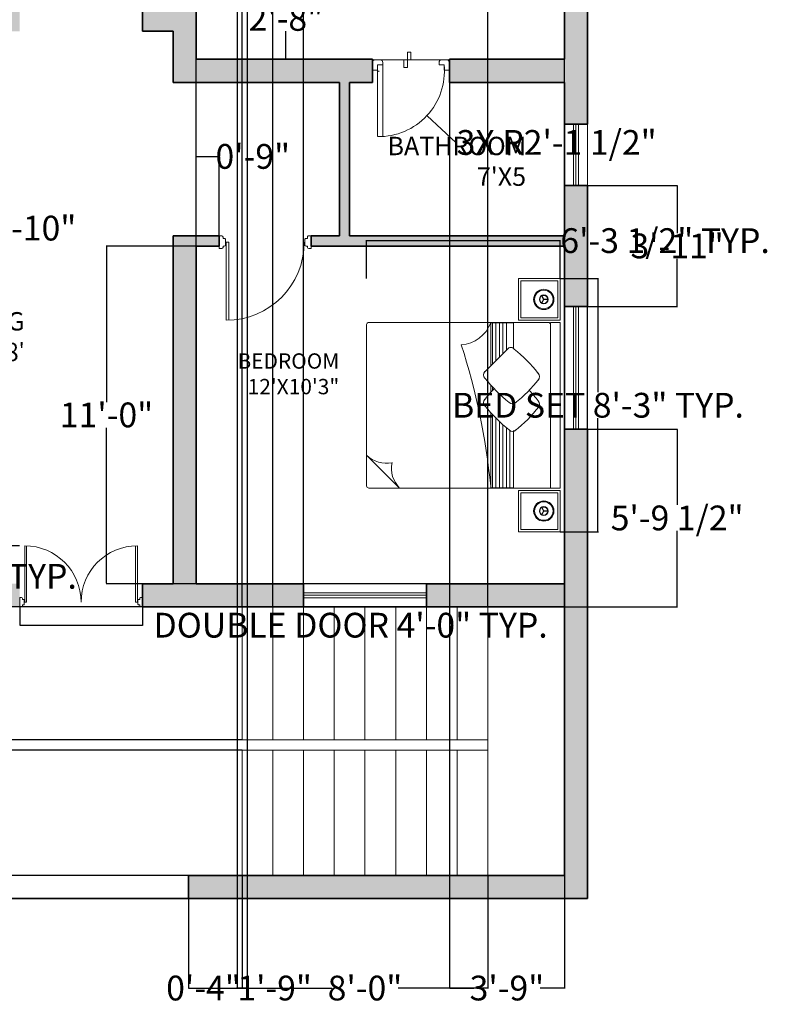
# Model space of a CAD drawing. Units: inches. Extents: x 2103 to 2702, y 2405 to 3142.
# Tile 2 of 7: x 2384 to 2677, y 2405 to 2790. Entities that reach past the tile are written whole.
import ezdxf

# ---------------------------------------------------------------- set-up
doc = ezdxf.new("R2010")
doc.units = ezdxf.units.IN
doc.linetypes.add('0', pattern=[0])
for name, color, linetype, lineweight in [('00 FURNITURE', 15, 'Continuous', 15), ('A-ANNO-DIMS', 2, 'Continuous', 18), ('A-AREA-IDEN', 7, 'Continuous', 18), ('A-FLOR-STRS', 7, 'Continuous', 18), ('A-WALL-PATT', 8, 'Continuous', 9), ('A_FUR 1', 5, 'Continuous', 5), ('doors', 4, 'Continuous', 18), ('WALL', 7, 'Continuous', 35), ('WINDOW', 160, '0', 5), ('windows', 4, 'Continuous', 18)]:
    doc.layers.add(name, color=color, linetype=linetype, lineweight=lineweight)
doc.layers.add('furniture', color=34, linetype='Continuous')
doc.styles.get("Standard").update_dxf_attribs({"font": 'arial.ttf'})
doc.dimstyles.get("Standard").update_dxf_attribs({"dimtxt": 9.68, "dimasz": 0.18, "dimexe": 0.18, "dimexo": 0.0625, "dimgap": 0.09, "dimtad": 0, "dimtih": 1, "dimtoh": 1, "dimdec": 1, "dimzin": 0, "dimdsep": 46, "dimlunit": 3, "dimtxsty": 'Standard', "dimcen": 0.09, "dimadec": 0, "dimazin": 0, "dimtfac": 1, "dimtdec": 1, "dimtofl": 0, "dimtmove": 0, "dimatfit": 3, "dimfxl": 1, "dimtolj": 1, "dimtzin": 0, "dimarcsym": 0})

# ---------------------------------------------------------------- blocks, each defined once
blk = doc.blocks.new('ESTSET')
at = {"layer": 'A_FUR 1'}
for p, q in [((-10.44, 4.1), (-10.44, 32.1)), ((-8.44, 4.1), (-8.44, 32.1)), ((-36.44, 6.1), (-36.44, 3.1)), ((-34.44, 6.1), (-36.44, 6.1)), ((-34.44, 4.1), (-34.44, 6.1)), ((-34.44, 4.1), (-34.44, 6.1)), ((-32.44, 4.1), (-34.44, 4.1)), ((-32.44, 4.1), (-34.44, 4.1)), ((-32.44, 3.1), (-32.44, 4.1)), ((-10.44, 3.1), (-10.44, 4.1)), ((-10.44, 4.1), (-8.44, 4.1)), ((-10.44, 4.1), (-8.44, 4.1)), ((-8.44, 4.1), (-8.44, 6.1)), ((-8.44, 6.1), (-6.44, 6.1)), ((-8.44, 4.1), (-8.44, 6.1)), ((-6.44, 6.1), (-6.44, 3.1)), ((-6.44, 2.1), (-36.44, 2.1)), ((-35.44, 2.1), (-33.44, 2.1)), ((-7.44, 2.1), (-9.44, 2.1))]:
    blk.add_line(p, q, dxfattribs=at)
for points in [[(-21.44, 2.1), (-18.67, 2.1), (-18.67, 5.1), (-20.06, 5.1)], [(-20.06, 5.1), (-20.06, -0.91)], [(-21.44, 2.1), (-21.44, -0.91), (-20.06, -0.91)]]:
    blk.add_lwpolyline(points, dxfattribs=at)
for centre, radius, start, end in [((-8.91, 6.46), 25.64, 88.9606, 185.2816), ((-35.44, 3.1), 1, 180, 270), ((-33.44, 3.1), 1, 270, 0), ((-9.44, 3.1), 1, 180, 270), ((-7.44, 3.1), 1, 270, 0)]:
    blk.add_arc(centre, radius, start, end, dxfattribs=at)
blk = doc.blocks.new('PUJA')
at = {"layer": '00 FURNITURE'}
for p, q in [((-1940.35, -16093.35), (-1958.14, -16093.35)), ((-1940.35, -16093.93), (-1958.13, -16093.93)), ((-1941.8, -16091.75), (-1938.89, -16091.75)), ((-1941.8, -16092.33), (-1941.8, -16091.75)), ((-1941.22, -16092.62), (-1941.51, -16092.62)), ((-1940.35, -16093.35), (-1940.35, -16093.93)), ((-1939.18, -16092.62), (-1939.47, -16092.62)), ((-1938.89, -16091.75), (-1938.89, -16092.33)), ((-1940.35, -16128.35), (-1958.13, -16128.35)), ((-1940.35, -16128.93), (-1940.35, -16128.35)), ((-1940.35, -16128.93), (-1958.14, -16128.93)), ((-1941.8, -16129.96), (-1941.8, -16130.54)), ((-1941.8, -16130.54), (-1938.89, -16130.54)), ((-1941.22, -16129.66), (-1941.51, -16129.66)), ((-1939.18, -16129.66), (-1939.47, -16129.66)), ((-1938.89, -16130.54), (-1938.89, -16129.96))]:
    blk.add_line(p, q, dxfattribs=at)
for points in [[(-1939.47, -16092.62), (-1939.47, -16092.91, -0.414214), (-1939.76, -16093.21), (-1940.93, -16093.21, -0.414214), (-1941.22, -16092.91), (-1941.22, -16092.62)], [(-1939.47, -16129.66), (-1939.47, -16129.37, 0.414214), (-1939.76, -16129.08), (-1940.93, -16129.08, 0.414214), (-1941.22, -16129.37), (-1941.22, -16129.66)]]:
    blk.add_lwpolyline(points, format="xyb", dxfattribs=at)
for centre, radius, start, end in [((-1940.35, -16093.35), 17.79, 180, 270), ((-1941.51, -16092.33), 0.292, 180, 270), ((-1939.18, -16092.33), 0.292, 270, 0), ((-1940.35, -16128.93), 17.79, 90, 180), ((-1941.51, -16129.96), 0.292, 90, 180), ((-1939.18, -16129.96), 0.292, 0, 90)]:
    blk.add_arc(centre, radius, start, end, dxfattribs=at)
blk = doc.blocks.new('DDD')
at = {"layer": '00 FURNITURE'}
for p, q in [((-12579.77, -15859.53), (-12579.77, -15829.05)), ((-12578.77, -15859.53), (-12578.77, -15829.03)), ((-12612.02, -15857.03), (-12612.02, -15862.03)), ((-12611.02, -15857.03), (-12612.02, -15857.03)), ((-12610.52, -15858.03), (-12610.52, -15857.53)), ((-12577.52, -15858.03), (-12577.52, -15857.53)), ((-12577.02, -15857.03), (-12576.02, -15857.03)), ((-12576.02, -15857.03), (-12576.02, -15862.03)), ((-12610.52, -15861.53), (-12610.52, -15861.03)), ((-12578.77, -15859.53), (-12579.77, -15859.53)), ((-12577.52, -15861.53), (-12577.52, -15861.03)), ((-12612.02, -15862.03), (-12611.02, -15862.03)), ((-12576.02, -15862.03), (-12577.02, -15862.03))]:
    blk.add_line(p, q, dxfattribs=at)
for points in [[(-12610.52, -15861.03), (-12610.02, -15861.03, 0.414214), (-12609.52, -15860.53), (-12609.52, -15858.53, 0.414214), (-12610.02, -15858.03), (-12610.52, -15858.03)], [(-12577.52, -15861.03), (-12578.02, -15861.03, -0.414214), (-12578.52, -15860.53), (-12578.52, -15858.53, -0.414214), (-12578.02, -15858.03), (-12577.52, -15858.03)]]:
    blk.add_lwpolyline(points, format="xyb", dxfattribs=at)
for centre, radius, start, end in [((-12578.77, -15859.53), 30.5, 90, 180), ((-12611.02, -15857.53), 0.5, 0, 90), ((-12577.02, -15857.53), 0.5, 90, 180), ((-12611.02, -15861.53), 0.5, 270, 0), ((-12577.02, -15861.53), 0.5, 180, 270)]:
    blk.add_arc(centre, radius, start, end, dxfattribs=at)
blk = doc.blocks.new('window')
at = {"layer": 'furniture'}
for p, q in [((1745.13, 2764.08), (1745.13, 2716.08)), ((1754.13, 2716.08), (1754.13, 2764.08))]:
    blk.add_line(p, q, dxfattribs=at)
at = {"layer": 'WINDOW'}
for p, q in [((1748.63, 2764.08), (1748.63, 2716.08)), ((1749.63, 2764.08), (1749.63, 2716.08)), ((1750.63, 2764.08), (1750.63, 2716.08))]:
    blk.add_line(p, q, dxfattribs=at)
blk = doc.blocks.new('ventilator')
at = {"layer": 'windows'}
for p, q in [((1922.12, 2523.05), (1898.12, 2523.05)), ((1922.12, 2522.05), (1898.12, 2522.05)), ((1922.12, 2521.05), (1898.12, 2521.05))]:
    blk.add_line(p, q, dxfattribs=at)
blk.add_lwpolyline([(1898.12, 2526.55), (1898.12, 2517.55), (1922.12, 2517.55), (1922.12, 2526.55)], close=True, dxfattribs=at)
blk = doc.blocks.new('RGWTG')
at = {"layer": '00 FURNITURE'}
for p, q in [((578.23, 3473.51), (577.36, 3475.01)), ((578.23, 3473.58), (577.36, 3472.08)), ((578.36, 3473.58), (577.49, 3475.09)), ((578.36, 3473.51), (577.49, 3472)), ((578.29, 3473.62), (580.03, 3473.62)), ((578.29, 3473.47), (580.03, 3473.47)), ((521.93, 3464.58), (509.03, 3451.68)), ((509.93, 3464.58), (566.4, 3464.58)), ((557.53, 3463.84), (557.53, 3464.49)), ((557.53, 3464.49), (566.4, 3464.49)), ((558.2, 3464.49), (558.2, 3435.82)), ((559.57, 3464.49), (559.57, 3437.25)), ((560.94, 3464.49), (560.94, 3438.58)), ((562.3, 3464.49), (562.3, 3439.83)), ((563.67, 3464.49), (563.67, 3440.99)), ((565.04, 3464.49), (565.04, 3442.08)), ((566.4, 3464.58), (580.98, 3464.58)), ((566.4, 3464.49), (566.4, 3442.08)), ((566.4, 3464.49), (566.4, 3463.84)), ((580.98, 3464.58), (580.98, 3416.72)), ((509.03, 3422.63), (509.03, 3463.68)), ((558.2, 3426.48), (558.2, 3425.04)), ((509.03, 3400.68), (509.03, 3422.63)), ((558.2, 3416.13), (558.2, 3399.95)), ((559.57, 3414.75), (559.57, 3399.95)), ((580.98, 3416.72), (580.98, 3400.68)), ((560.94, 3413.39), (560.94, 3399.95)), ((562.3, 3412.04), (562.3, 3399.95)), ((563.67, 3410.72), (563.67, 3399.95)), ((580.08, 3399.78), (509.93, 3399.78)), ((557.53, 3399.95), (557.53, 3400.6)), ((566.4, 3399.95), (557.53, 3399.95)), ((566.4, 3400.6), (566.4, 3399.95)), ((578.23, 3390.78), (577.36, 3392.29)), ((578.36, 3390.86), (577.49, 3392.36)), ((578.23, 3390.86), (577.36, 3389.36)), ((578.36, 3390.78), (577.49, 3389.28)), ((578.29, 3390.9), (580.03, 3390.9)), ((578.29, 3390.74), (580.03, 3390.74))]:
    blk.add_line(p, q, dxfattribs=at)
for points in [[(568.43, 3465.48), (584.63, 3465.48), (584.63, 3481.68), (568.43, 3481.68)], [(569.33, 3466.38), (583.73, 3466.38), (583.73, 3480.78), (569.33, 3480.78)], [(580.98, 3399.78), (584.63, 3399.78), (584.63, 3464.58), (580.98, 3464.58)], [(568.43, 3398.88), (584.63, 3398.88), (584.63, 3382.68), (568.43, 3382.68)], [(569.33, 3397.98), (583.73, 3397.98), (583.73, 3383.58), (569.33, 3383.58)]]:
    blk.add_lwpolyline(points, close=True, dxfattribs=at)
for points in [[(566.52, 3464.49), (557.53, 3464.49), (557.53, 3435.08)], [(557.53, 3427.21), (557.53, 3424.3)], [(557.53, 3416.82), (557.53, 3399.95), (566.4, 3399.95), (566.4, 3409.94)]]:
    blk.add_lwpolyline(points, dxfattribs=at)
for centre, radius in [((578.29, 3473.54), 3.97), ((578.29, 3473.54), 3.63), ((578.29, 3473.54), 1.74), ((578.29, 3473.54), 1.56), ((578.29, 3390.82), 3.97), ((578.29, 3390.82), 3.63), ((578.29, 3390.82), 1.74), ((578.29, 3390.82), 1.56)]:
    blk.add_circle(centre, radius, dxfattribs=at)
for centre, radius, start, end in [((509.93, 3463.68), 0.9, 90, 180), ((529.65, 3456.88), 10.9, 135.0361, 191.9278), ((290.56, 3490.52), 268.3, 342.2214, 354.2925), ((516.73, 3443.97), 10.9, 78.0722, 134.9639), ((598.15, 3399.01), 54.32, 127.931, 142.069), ((566.05, 3440.57), 1.82, 45, 135), ((533.58, 3399.31), 54.32, 37.931, 52.069), ((556.59, 3431.11), 1.82, 135, 225), ((597.87, 3463.6), 54.32, 217.931, 224.141), ((598.15, 3388.23), 54.32, 127.931, 142.069), ((566.05, 3429.78), 1.82, 45, 135), ((533.58, 3388.53), 54.32, 37.931, 52.069), ((533.28, 3463.88), 54.32, 316.32, 322.069), ((574.84, 3431.77), 1.82, 315, 45), ((574.84, 3420.99), 1.82, 315, 45), ((556.59, 3420.33), 1.82, 135, 225), ((765.33, 3619.75), 290.45, 223.6069, 226.2326), ((533.28, 3453.1), 54.32, 307.931, 322.069), ((565.44, 3411.05), 1.47, 225.9674, 326.8337), ((545.02, 3395.29), 13.35, 20.4224, 85.5825), ((509.93, 3400.68), 0.9, 180, 270), ((580.08, 3400.68), 0.9, 270, 0)]:
    blk.add_arc(centre, radius, start, end, dxfattribs=at)
blk = doc.blocks.new('*D26')
at = {"layer": 'A-ANNO-DIMS', "color": 0, "lineweight": -2, "transparency": 16777216}
for p, q in [((2384.43, 2560.78), (2384.43, 2553.47)), ((2432.43, 2560.78), (2432.43, 2553.47)), ((2384.61, 2553.65), (2432.25, 2553.65)), ((2432.43, 2553.65), (2432.61, 2553.65))]:
    blk.add_line(p, q, dxfattribs=at)
at = {"layer": 'A-ANNO-DIMS', "color": 0, "transparency": 16777216}
for points in [[(2384.61, 2553.68), (2384.61, 2553.62), (2384.43, 2553.65)], [(2432.25, 2553.68), (2432.25, 2553.62), (2432.43, 2553.65)]]:
    blk.add_solid(points, dxfattribs=at)
at = {"layer": 'Defpoints', "color": 0, "transparency": 16777216}
for p in [(2384.43, 2560.85), (2432.43, 2560.85), (2432.43, 2553.65)]:
    blk.add_point(p, dxfattribs=at)
at = {"layer": 'A-ANNO-DIMS', "color": 0, "transparency": 16777216, "insert": (2513.81, 2553.65), "char_height": 9.68, "attachment_point": 5}
blk.add_mtext('\\A1;DOUBLE DOOR 4\'-0" TYP.', dxfattribs=at)
blk = doc.blocks.new('*D27')
at = {"layer": 'A-ANNO-DIMS', "color": 0, "lineweight": -2, "transparency": 16777216}
for p, q in [((2384.37, 2584.67), (2377.05, 2584.67)), ((2377.23, 2584.49), (2377.23, 2577.79)), ((2377.23, 2561.03), (2377.23, 2567.72)), ((2384.37, 2560.85), (2377.05, 2560.85))]:
    blk.add_line(p, q, dxfattribs=at)
at = {"layer": 'A-ANNO-DIMS', "color": 0, "transparency": 16777216}
for points in [[(2377.2, 2584.49), (2377.26, 2584.49), (2377.23, 2584.67)], [(2377.2, 2561.03), (2377.26, 2561.03), (2377.23, 2560.85)]]:
    blk.add_solid(points, dxfattribs=at)
at = {"layer": 'Defpoints', "color": 0, "transparency": 16777216}
for p in [(2384.43, 2584.67), (2377.23, 2560.85), (2384.43, 2560.85)]:
    blk.add_point(p, dxfattribs=at)
at = {"layer": 'A-ANNO-DIMS', "color": 0, "transparency": 16777216, "insert": (2377.23, 2572.76), "char_height": 9.68, "attachment_point": 5}
blk.add_mtext('\\A1;2\'-0" TYP.', dxfattribs=at)
blk = doc.blocks.new('*D28')
at = {"layer": 'A-ANNO-DIMS', "color": 0, "lineweight": -2, "transparency": 16777216}
for p, q in [((2595.74, 2689.13), (2610.71, 2689.13)), ((2610.53, 2688.95), (2610.53, 2644.73)), ((2610.53, 2590.31), (2610.53, 2634.53)), ((2595.74, 2590.13), (2610.71, 2590.13))]:
    blk.add_line(p, q, dxfattribs=at)
at = {"layer": 'A-ANNO-DIMS', "color": 0, "transparency": 16777216}
for points in [[(2610.5, 2688.95), (2610.56, 2688.95), (2610.53, 2689.13)], [(2610.5, 2590.31), (2610.56, 2590.31), (2610.53, 2590.13)]]:
    blk.add_solid(points, dxfattribs=at)
at = {"layer": 'Defpoints', "color": 0, "transparency": 16777216}
for p in [(2595.68, 2689.13), (2595.68, 2590.13), (2610.53, 2590.13)]:
    blk.add_point(p, dxfattribs=at)
at = {"layer": 'A-ANNO-DIMS', "color": 0, "transparency": 16777216, "insert": (2610.53, 2639.63), "char_height": 9.68, "attachment_point": 5}
blk.add_mtext('\\A1;BED SET 8\'-3" TYP.', dxfattribs=at)
blk = doc.blocks.new('*D29')
at = {"layer": 'A-ANNO-DIMS', "color": 0, "lineweight": -2, "transparency": 16777216}
for p, q in [((2520.08, 2689.19), (2520.08, 2704.16)), ((2520.26, 2703.98), (2595.5, 2703.98)), ((2595.68, 2689.19), (2595.68, 2704.16)), ((2595.68, 2703.98), (2595.86, 2703.98))]:
    blk.add_line(p, q, dxfattribs=at)
at = {"layer": 'A-ANNO-DIMS', "color": 0, "transparency": 16777216}
for points in [[(2520.26, 2704.01), (2520.26, 2703.95), (2520.08, 2703.98)], [(2595.5, 2704.01), (2595.5, 2703.95), (2595.68, 2703.98)]]:
    blk.add_solid(points, dxfattribs=at)
at = {"layer": 'Defpoints', "color": 0, "transparency": 16777216}
for p in [(2595.68, 2703.98), (2520.08, 2689.13), (2595.68, 2689.13)]:
    blk.add_point(p, dxfattribs=at)
at = {"layer": 'A-ANNO-DIMS', "color": 0, "transparency": 16777216, "insert": (2636.76, 2703.98), "char_height": 9.68, "attachment_point": 5}
blk.add_mtext('\\A1;6\'-3 1/2" TYP.', dxfattribs=at)
blk = doc.blocks.new('*D41')
at = {"layer": 'A-ANNO-DIMS', "color": 0, "lineweight": -2, "transparency": 16777216}
for p, q in [((2471.43, 2455.78), (2471.43, 2411.62)), ((2567.43, 2455.78), (2567.43, 2411.62)), ((2471.61, 2411.8), (2506.47, 2411.8)), ((2567.25, 2411.8), (2532.39, 2411.8))]:
    blk.add_line(p, q, dxfattribs=at)
at = {"layer": 'A-ANNO-DIMS', "color": 0, "transparency": 16777216}
for points in [[(2471.61, 2411.83), (2471.61, 2411.77), (2471.43, 2411.8)], [(2567.25, 2411.83), (2567.25, 2411.77), (2567.43, 2411.8)]]:
    blk.add_solid(points, dxfattribs=at)
at = {"layer": 'Defpoints', "color": 0, "transparency": 16777216}
for p in [(2471.43, 2455.85), (2567.43, 2455.85), (2567.43, 2411.8)]:
    blk.add_point(p, dxfattribs=at)
at = {"layer": 'A-ANNO-DIMS', "color": 0, "transparency": 16777216, "insert": (2519.43, 2411.8), "char_height": 9.68, "attachment_point": 5}
blk.add_mtext('\\A1;8\'-0"', dxfattribs=at)
blk = doc.blocks.new('*D42')
at = {"layer": 'A-ANNO-DIMS', "color": 0, "lineweight": -2, "transparency": 16777216}
for p, q in [((2471.37, 2504.85), (2211.2, 2504.85)), ((2211.38, 2504.67), (2211.38, 2485.3)), ((2211.38, 2456.03), (2211.38, 2475.4)), ((2471.37, 2455.85), (2211.2, 2455.85))]:
    blk.add_line(p, q, dxfattribs=at)
at = {"layer": 'A-ANNO-DIMS', "color": 0, "transparency": 16777216}
for points in [[(2211.35, 2504.67), (2211.41, 2504.67), (2211.38, 2504.85)], [(2211.35, 2456.03), (2211.41, 2456.03), (2211.38, 2455.85)]]:
    blk.add_solid(points, dxfattribs=at)
at = {"layer": 'Defpoints', "color": 0, "transparency": 16777216}
for p in [(2211.38, 2504.85), (2471.43, 2504.85), (2471.43, 2455.85)]:
    blk.add_point(p, dxfattribs=at)
at = {"layer": 'A-ANNO-DIMS', "color": 0, "transparency": 16777216, "insert": (2211.38, 2480.35), "char_height": 9.68, "attachment_point": 5}
blk.add_mtext('\\A1;4\'-1"', dxfattribs=at)
blk = doc.blocks.new('*D43')
at = {"layer": 'A-ANNO-DIMS', "color": 0, "lineweight": -2, "transparency": 16777216}
for p, q in [((2471.367635, 2560.845674), (2211.200134, 2560.845674)), ((2211.380134, 2560.665674), (2211.380134, 2539.775674)), ((2211.380134, 2509.025674), (2211.380134, 2529.915674)), ((2471.367635, 2508.845674), (2211.200134, 2508.845674))]:
    blk.add_line(p, q, dxfattribs=at)
at = {"layer": 'A-ANNO-DIMS', "color": 0, "transparency": 16777216}
for points in [[(2211.350134, 2560.665674), (2211.410134, 2560.665674), (2211.380134, 2560.845674)], [(2211.350134, 2509.025674), (2211.410134, 2509.025674), (2211.380134, 2508.845674)]]:
    blk.add_solid(points, dxfattribs=at)
at = {"layer": 'Defpoints', "color": 0, "transparency": 16777216}
for p in [(2211.380134, 2560.845674), (2471.430135, 2560.845674), (2471.430135, 2508.845674)]:
    blk.add_point(p, dxfattribs=at)
at = {"layer": 'A-ANNO-DIMS', "color": 0, "transparency": 16777216, "insert": (2211.380134, 2534.845674), "char_height": 9.68, "attachment_point": 5}
blk.add_mtext('\\A1;4\'-4"', dxfattribs=at)
blk = doc.blocks.new('*D44')
at = {"layer": 'A-ANNO-DIMS', "color": 0, "lineweight": -2, "transparency": 16777216}
for p, q in [((2471.43, 2560.91), (2471.43, 3118.9)), ((2471.61, 3118.72), (2483.25, 3118.72)), ((2483.43, 2560.91), (2483.43, 3118.9)), ((2483.43, 3118.72), (2483.61, 3118.72))]:
    blk.add_line(p, q, dxfattribs=at)
at = {"layer": 'A-ANNO-DIMS', "color": 0, "transparency": 16777216}
for points in [[(2471.61, 3118.75), (2471.61, 3118.69), (2471.43, 3118.72)], [(2483.25, 3118.75), (2483.25, 3118.69), (2483.43, 3118.72)]]:
    blk.add_solid(points, dxfattribs=at)
at = {"layer": 'Defpoints', "color": 0, "transparency": 16777216}
for p in [(2483.43, 3118.72), (2471.43, 2560.85), (2483.43, 2560.85)]:
    blk.add_point(p, dxfattribs=at)
at = {"layer": 'A-ANNO-DIMS', "color": 0, "transparency": 16777216, "insert": (2496.11, 3118.72), "char_height": 9.68, "attachment_point": 5}
blk.add_mtext('\\A1;1\'-0"', dxfattribs=at)
blk = doc.blocks.new('*D45')
at = {"layer": 'A-ANNO-DIMS', "color": 0, "lineweight": -2, "transparency": 16777216}
for p, q in [((2567.43, 2560.91), (2567.43, 3118.9)), ((2567.61, 3118.72), (2569.39, 3118.72)), ((2597.25, 3118.72), (2595.47, 3118.72)), ((2597.43, 2560.91), (2597.43, 3118.9))]:
    blk.add_line(p, q, dxfattribs=at)
at = {"layer": 'A-ANNO-DIMS', "color": 0, "transparency": 16777216}
for points in [[(2567.61, 3118.75), (2567.61, 3118.69), (2567.43, 3118.72)], [(2597.25, 3118.75), (2597.25, 3118.69), (2597.43, 3118.72)]]:
    blk.add_solid(points, dxfattribs=at)
at = {"layer": 'Defpoints', "color": 0, "transparency": 16777216}
for p in [(2597.43, 3118.72), (2567.43, 2560.85), (2597.43, 2560.85)]:
    blk.add_point(p, dxfattribs=at)
at = {"layer": 'A-ANNO-DIMS', "color": 0, "transparency": 16777216, "insert": (2582.43, 3118.72), "char_height": 9.68, "attachment_point": 5}
blk.add_mtext('\\A1;2\'-6"', dxfattribs=at)
blk = doc.blocks.new('*D46')
at = {"layer": 'A-ANNO-DIMS', "color": 0, "lineweight": -2, "transparency": 16777216}
for p, q in [((2450.43, 2455.78), (2450.43, 2411.62)), ((2471.43, 2455.78), (2471.43, 2411.62)), ((2450.61, 2411.8), (2471.25, 2411.8)), ((2471.43, 2411.8), (2471.61, 2411.8))]:
    blk.add_line(p, q, dxfattribs=at)
at = {"layer": 'A-ANNO-DIMS', "color": 0, "transparency": 16777216}
for points in [[(2450.61, 2411.83), (2450.61, 2411.77), (2450.43, 2411.8)], [(2471.25, 2411.83), (2471.25, 2411.77), (2471.43, 2411.8)]]:
    blk.add_solid(points, dxfattribs=at)
at = {"layer": 'Defpoints', "color": 0, "transparency": 16777216}
for p in [(2450.43, 2455.85), (2471.43, 2455.85), (2471.43, 2411.8)]:
    blk.add_point(p, dxfattribs=at)
at = {"layer": 'A-ANNO-DIMS', "color": 0, "transparency": 16777216, "insert": (2484.11, 2411.8), "char_height": 9.68, "attachment_point": 5}
blk.add_mtext('\\A1;1\'-9"', dxfattribs=at)
blk = doc.blocks.new('*D47')
at = {"layer": 'A-ANNO-DIMS', "color": 0, "lineweight": -2, "transparency": 16777216}
for p, q in [((2471.37, 2508.85), (2211.2, 2508.85)), ((2211.38, 2508.85), (2211.38, 2509.03)), ((2211.38, 2509.03), (2211.56, 2509.03)), ((2211.38, 2505.03), (2211.38, 2508.67)), ((2471.37, 2504.85), (2211.2, 2504.85))]:
    blk.add_line(p, q, dxfattribs=at)
at = {"layer": 'A-ANNO-DIMS', "color": 0, "transparency": 16777216}
for points in [[(2211.35, 2508.67), (2211.41, 2508.67), (2211.38, 2508.85)], [(2211.35, 2505.03), (2211.41, 2505.03), (2211.38, 2504.85)]]:
    blk.add_solid(points, dxfattribs=at)
at = {"layer": 'Defpoints', "color": 0, "transparency": 16777216}
for p in [(2211.38, 2508.85), (2471.43, 2508.85), (2471.43, 2504.85)]:
    blk.add_point(p, dxfattribs=at)
at = {"layer": 'A-ANNO-DIMS', "color": 0, "transparency": 16777216, "insert": (2224.52, 2509.03), "char_height": 9.68, "attachment_point": 5}
blk.add_mtext('\\A1;0\'-4"', dxfattribs=at)
blk = doc.blocks.new('*D50')
at = {"layer": 'A-ANNO-DIMS', "color": 0, "lineweight": -2, "transparency": 16777216}
for p, q in [((2453.43, 2569.91), (2453.43, 3118.9)), ((2453.61, 3118.72), (2461.48, 3118.72)), ((2495.25, 3118.72), (2487.38, 3118.72)), ((2495.43, 2569.91), (2495.43, 3118.9))]:
    blk.add_line(p, q, dxfattribs=at)
at = {"layer": 'A-ANNO-DIMS', "color": 0, "transparency": 16777216}
for points in [[(2453.61, 3118.75), (2453.61, 3118.69), (2453.43, 3118.72)], [(2495.25, 3118.75), (2495.25, 3118.69), (2495.43, 3118.72)]]:
    blk.add_solid(points, dxfattribs=at)
at = {"layer": 'Defpoints', "color": 0, "transparency": 16777216}
for p in [(2495.43, 3118.72), (2453.43, 2569.85), (2495.43, 2569.85)]:
    blk.add_point(p, dxfattribs=at)
at = {"layer": 'A-ANNO-DIMS', "color": 0, "transparency": 16777216, "insert": (2474.43, 3118.72), "char_height": 9.68, "attachment_point": 5}
blk.add_mtext('\\A1;3\'-6"', dxfattribs=at)
blk = doc.blocks.new('*D61')
at = {"layer": 'A-ANNO-DIMS', "color": 0, "lineweight": -2, "transparency": 16777216}
for p, q in [((2606.49, 2630.29), (2641.66, 2630.29)), ((2641.48, 2630.11), (2641.48, 2600.66)), ((2641.48, 2561.03), (2641.48, 2590.47)), ((2597.49, 2560.85), (2641.66, 2560.85))]:
    blk.add_line(p, q, dxfattribs=at)
at = {"layer": 'A-ANNO-DIMS', "color": 0, "transparency": 16777216}
for points in [[(2641.45, 2630.11), (2641.51, 2630.11), (2641.48, 2630.29)], [(2641.45, 2561.03), (2641.51, 2561.03), (2641.48, 2560.85)]]:
    blk.add_solid(points, dxfattribs=at)
at = {"layer": 'Defpoints', "color": 0, "transparency": 16777216}
for p in [(2606.43, 2630.29), (2641.48, 2630.29), (2597.43, 2560.85)]:
    blk.add_point(p, dxfattribs=at)
at = {"layer": 'A-ANNO-DIMS', "color": 0, "transparency": 16777216, "insert": (2641.48, 2595.57), "char_height": 9.68, "attachment_point": 5}
blk.add_mtext('\\A1;5\'-9 1/2"', dxfattribs=at)
blk = doc.blocks.new('*D62')
at = {"layer": 'A-ANNO-DIMS', "color": 0, "lineweight": -2, "transparency": 16777216}
for p, q in [((2606.49, 2725.52), (2641.66, 2725.52)), ((2641.48, 2725.34), (2641.48, 2706.94)), ((2641.48, 2678.47), (2641.48, 2696.87)), ((2606.49, 2678.29), (2641.66, 2678.29))]:
    blk.add_line(p, q, dxfattribs=at)
at = {"layer": 'A-ANNO-DIMS', "color": 0, "transparency": 16777216}
for points in [[(2641.45, 2725.34), (2641.51, 2725.34), (2641.48, 2725.52)], [(2641.45, 2678.47), (2641.51, 2678.47), (2641.48, 2678.29)]]:
    blk.add_solid(points, dxfattribs=at)
at = {"layer": 'Defpoints', "color": 0, "transparency": 16777216}
for p in [(2606.43, 2725.52), (2641.48, 2725.52), (2606.43, 2678.29)]:
    blk.add_point(p, dxfattribs=at)
at = {"layer": 'A-ANNO-DIMS', "color": 0, "transparency": 16777216, "insert": (2641.48, 2701.91), "char_height": 9.68, "attachment_point": 5}
blk.add_mtext('\\A1;3\'-11"', dxfattribs=at)
blk = doc.blocks.new('*D67')
at = {"layer": 'A-ANNO-DIMS', "color": 0, "lineweight": -2, "transparency": 16777216}
for p, q in [((2469.43, 2999.78), (2469.43, 2411.62)), ((2473.43, 2999.78), (2473.43, 2411.62)), ((2469.43, 2411.8), (2469.25, 2411.8)), ((2473.25, 2411.8), (2469.61, 2411.8))]:
    blk.add_line(p, q, dxfattribs=at)
at = {"layer": 'A-ANNO-DIMS', "color": 0, "transparency": 16777216}
for points in [[(2469.61, 2411.83), (2469.61, 2411.77), (2469.43, 2411.8)], [(2473.25, 2411.83), (2473.25, 2411.77), (2473.43, 2411.8)]]:
    blk.add_solid(points, dxfattribs=at)
at = {"layer": 'Defpoints', "color": 0, "transparency": 16777216}
for p in [(2469.43, 2999.85), (2473.43, 2999.85), (2469.43, 2411.8)]:
    blk.add_point(p, dxfattribs=at)
at = {"layer": 'A-ANNO-DIMS', "color": 0, "transparency": 16777216, "insert": (2456.29, 2411.8), "char_height": 9.68, "attachment_point": 5}
blk.add_mtext('\\A1;0\'-4"', dxfattribs=at)
blk = doc.blocks.new('*D71')
at = {"layer": 'A-ANNO-DIMS', "color": 0, "lineweight": -2, "transparency": 16777216}
for p, q in [((2453.49, 2806.85), (2488.66, 2806.85)), ((2488.48, 2806.67), (2488.48, 2795.88)), ((2488.48, 2775.03), (2488.48, 2785.81)), ((2453.49, 2774.85), (2488.66, 2774.85))]:
    blk.add_line(p, q, dxfattribs=at)
at = {"layer": 'A-ANNO-DIMS', "color": 0, "transparency": 16777216}
for points in [[(2488.45, 2806.67), (2488.51, 2806.67), (2488.48, 2806.85)], [(2488.45, 2775.03), (2488.51, 2775.03), (2488.48, 2774.85)]]:
    blk.add_solid(points, dxfattribs=at)
at = {"layer": 'Defpoints', "color": 0, "transparency": 16777216}
for p in [(2453.43, 2806.85), (2453.43, 2774.85), (2488.48, 2774.85)]:
    blk.add_point(p, dxfattribs=at)
at = {"layer": 'A-ANNO-DIMS', "color": 0, "transparency": 16777216, "insert": (2488.48, 2790.85), "char_height": 9.68, "attachment_point": 5}
blk.add_mtext('\\A1;2\'-8"', dxfattribs=at)
blk = doc.blocks.new('*D72')
at = {"layer": 'A-ANNO-DIMS', "color": 0, "lineweight": -2, "transparency": 16777216}
for p, q in [((2453.43, 2701.91), (2453.43, 2737.08)), ((2453.61, 2736.9), (2462.25, 2736.9)), ((2462.43, 2701.91), (2462.43, 2737.08)), ((2462.43, 2736.9), (2462.61, 2736.9))]:
    blk.add_line(p, q, dxfattribs=at)
at = {"layer": 'A-ANNO-DIMS', "color": 0, "transparency": 16777216}
for points in [[(2453.61, 2736.93), (2453.61, 2736.87), (2453.43, 2736.9)], [(2462.25, 2736.93), (2462.25, 2736.87), (2462.43, 2736.9)]]:
    blk.add_solid(points, dxfattribs=at)
at = {"layer": 'Defpoints', "color": 0, "transparency": 16777216}
for p in [(2462.43, 2736.9), (2453.43, 2701.85), (2462.43, 2701.85)]:
    blk.add_point(p, dxfattribs=at)
at = {"layer": 'A-ANNO-DIMS', "color": 0, "transparency": 16777216, "insert": (2475.57, 2736.9), "char_height": 9.68, "attachment_point": 5}
blk.add_mtext('\\A1;0\'-9"', dxfattribs=at)
blk = doc.blocks.new('*D73')
at = {"layer": 'A-ANNO-DIMS', "color": 0, "lineweight": -2, "transparency": 16777216}
for p, q in [((2552.43, 2765.78), (2552.43, 2411.62)), ((2597.43, 2765.78), (2597.43, 2411.62)), ((2552.61, 2411.8), (2561.98, 2411.8)), ((2597.25, 2411.8), (2587.88, 2411.8))]:
    blk.add_line(p, q, dxfattribs=at)
at = {"layer": 'A-ANNO-DIMS', "color": 0, "transparency": 16777216}
for points in [[(2552.61, 2411.83), (2552.61, 2411.77), (2552.43, 2411.8)], [(2597.25, 2411.83), (2597.25, 2411.77), (2597.43, 2411.8)]]:
    blk.add_solid(points, dxfattribs=at)
at = {"layer": 'Defpoints', "color": 0, "transparency": 16777216}
for p in [(2552.43, 2765.85), (2597.43, 2765.85), (2597.43, 2411.8)]:
    blk.add_point(p, dxfattribs=at)
at = {"layer": 'A-ANNO-DIMS', "color": 0, "transparency": 16777216, "insert": (2574.93, 2411.8), "char_height": 9.68, "attachment_point": 5}
blk.add_mtext('\\A1;3\'-9"', dxfattribs=at)
blk = doc.blocks.new('*D75')
at = {"layer": 'A-ANNO-DIMS', "color": 0, "lineweight": -2, "transparency": 16777216}
for p, q in [((2453.37, 2701.85), (2418.2, 2701.85)), ((2418.38, 2701.67), (2418.38, 2640.88)), ((2418.38, 2570.03), (2418.38, 2630.81)), ((2453.37, 2569.85), (2418.2, 2569.85))]:
    blk.add_line(p, q, dxfattribs=at)
at = {"layer": 'A-ANNO-DIMS', "color": 0, "transparency": 16777216}
for points in [[(2418.35, 2701.67), (2418.41, 2701.67), (2418.38, 2701.85)], [(2418.35, 2570.03), (2418.41, 2570.03), (2418.38, 2569.85)]]:
    blk.add_solid(points, dxfattribs=at)
at = {"layer": 'Defpoints', "color": 0, "transparency": 16777216}
for p in [(2418.38, 2701.85), (2453.43, 2701.85), (2453.43, 2569.85)]:
    blk.add_point(p, dxfattribs=at)
at = {"layer": 'A-ANNO-DIMS', "color": 0, "transparency": 16777216, "insert": (2418.38, 2635.85), "char_height": 9.68, "attachment_point": 5}
blk.add_mtext('\\A1;11\'-0"', dxfattribs=at)
blk = doc.blocks.new('*D78')
at = {"layer": 'A-ANNO-DIMS', "color": 0, "lineweight": -2, "transparency": 16777216}
for p, q in [((2342.12, 2708.86), (2342.3, 2708.86)), ((2342.21, 2708.77), (2342.21, 2708.95)), ((2359.73, 2708.87), (2353.34, 2708.86))]:
    blk.add_line(p, q, dxfattribs=at)
at = {"layer": 'A-ANNO-DIMS', "color": 0, "transparency": 16777216}
blk.add_solid([(2353.34, 2708.9), (2353.34, 2708.84), (2353.16, 2708.86)], dxfattribs=at)
at = {"layer": 'Defpoints', "color": 0, "transparency": 16777216}
for p in [(2331.26, 2708.86), (2353.16, 2708.86)]:
    blk.add_point(p, dxfattribs=at)
at = {"layer": 'A-ANNO-DIMS', "color": 0, "transparency": 16777216, "insert": (2381.71, 2708.87), "char_height": 9.68, "attachment_point": 5}
blk.add_mtext('\\A1;∅1\'-10"', dxfattribs=at)
blk = doc.blocks.new('*D80')
at = {"layer": 'A-ANNO-DIMS', "color": 0, "lineweight": -2, "transparency": 16777216}
for p, q in [((2524.77, 2770.28), (2524.95, 2770.28)), ((2524.86, 2770.19), (2524.86, 2770.37)), ((2554.93, 2742.36), (2543.79, 2752.71)), ((2555.11, 2742.36), (2554.93, 2742.36))]:
    blk.add_line(p, q, dxfattribs=at)
at = {"layer": 'A-ANNO-DIMS', "color": 0, "transparency": 16777216}
blk.add_solid([(2543.81, 2752.73), (2543.77, 2752.68), (2543.65, 2752.83)], dxfattribs=at)
at = {"layer": 'Defpoints', "color": 0, "transparency": 16777216}
for p in [(2524.86, 2770.28), (2543.65, 2752.83)]:
    blk.add_point(p, dxfattribs=at)
at = {"layer": 'A-ANNO-DIMS', "color": 0, "transparency": 16777216, "insert": (2594.37, 2742.36), "char_height": 9.68, "attachment_point": 5}
blk.add_mtext('\\A1;3X R2\'-1 1/2"', dxfattribs=at)

msp = doc.modelspace()

# ---------------------------------------------------------------- hatches: boundary and pattern name
at = {"layer": 'A-WALL-PATT'}
h = msp.add_hatch(color=256, dxfattribs=at)
h.dxf.hatch_style = 1
h.paths.add_polyline_path([(2342.43, 2911.85), (2342.43, 2915.85), (2255.43, 2915.85), (2255.43, 2976.23), (2246.43, 2976.23), (2246.43, 2840.19), (2255.43, 2840.19), (2255.43, 2854.85), (2315.43, 2854.85), (2315.43, 2845.85), (2319.43, 2845.85), (2319.43, 2858.85), (2255.43, 2858.85), (2255.43, 2906.85), (2342.43, 2906.85)])
h.paths.add_polyline_path([(2384.43, 2794.85), (2319.43, 2794.85), (2319.43, 2815.85), (2315.43, 2815.85), (2315.43, 2794.85), (2255.43, 2794.85), (2255.43, 2816.19), (2246.43, 2816.19), (2246.43, 2753.7), (2255.43, 2753.7), (2255.43, 2785.85), (2384.43, 2785.85)])
h.paths.add_polyline_path([(2606.43, 2963.85), (2597.43, 2963.85), (2597.43, 2951.85), (2537.43, 2951.85), (2537.43, 2957.85), (2533.43, 2957.85), (2533.43, 2951.85), (2469.43, 2951.85), (2444.43, 2951.85), (2444.43, 2842.85), (2449.43, 2842.85), (2453.43, 2842.85), (2453.43, 2942.85), (2597.43, 2942.85), (2597.43, 2904.89), (2606.43, 2904.89)])
h.paths.add_polyline_path([(2606.43, 3019.85), (2597.43, 3019.85), (2597.43, 3003.85), (2537.43, 3003.85), (2537.43, 3015.85), (2533.43, 3015.85), (2533.43, 2987.85), (2537.43, 2987.85), (2537.43, 2999.85), (2597.43, 2999.85), (2597.43, 2987.85), (2606.43, 2987.85)])
h.paths.add_polyline_path([(2606.43, 2856.89), (2597.43, 2856.89), (2597.43, 2774.85), (2552.43, 2774.85), (2552.43, 2765.85), (2597.43, 2765.85), (2597.43, 2749.52), (2606.43, 2749.52)])
h.paths.add_polyline_path([(2522.43, 2774.85), (2453.43, 2774.85), (2453.43, 2806.85), (2444.43, 2806.85), (2444.43, 2794.85), (2432.43, 2794.85), (2432.43, 2785.85), (2444.43, 2785.85), (2444.43, 2765.85), (2453.43, 2765.85), (2509.43, 2765.85), (2509.43, 2705.85), (2498.43, 2705.85), (2498.43, 2701.85), (2597.43, 2701.85), (2597.43, 2678.29), (2606.43, 2678.29), (2606.43, 2725.52), (2597.43, 2725.52), (2597.43, 2705.85), (2513.43, 2705.85), (2513.43, 2765.85), (2522.43, 2765.85)])
h.paths.add_polyline_path([(2255.43, 2705.7), (2246.43, 2705.7), (2246.43, 2646.55), (2255.43, 2646.55)])
h.paths.add_polyline_path([(2255.43, 2598.55), (2246.43, 2598.55), (2246.43, 2560.85), (2309.13, 2560.85), (2309.13, 2569.85), (2309.13, 2569.85), (2255.43, 2569.85)])
h.paths.add_polyline_path([(2495.43, 2569.85), (2495.43, 2569.85), (2453.43, 2569.85), (2453.43, 2701.85), (2462.43, 2701.85), (2462.43, 2705.85), (2444.43, 2705.85), (2444.43, 2569.85), (2432.43, 2569.85), (2432.43, 2564.45), (2432.43, 2564.45), (2432.43, 2560.85), (2495.43, 2560.85)])
h.paths.add_polyline_path([(2384.43, 2569.85), (2357.13, 2569.85), (2357.13, 2560.85), (2384.43, 2560.85)])
h.paths.add_polyline_path([(2606.43, 2630.29), (2597.43, 2630.29), (2597.43, 2569.85), (2543.43, 2569.85), (2543.43, 2560.85), (2597.43, 2560.85), (2597.43, 2455.85), (2450.43, 2455.85), (2450.43, 2446.85), (2606.43, 2446.85)])

# ---------------------------------------------------------------- linework, layer by layer
at = {"layer": 'A-FLOR-STRS'}
for p, q in [((2471.43, 2560.85), (2471.43, 2508.85)), ((2483.43, 2560.85), (2483.43, 2508.85)), ((2495.43, 2560.85), (2495.43, 2508.85)), ((2507.43, 2560.85), (2507.43, 2508.85)), ((2519.43, 2560.85), (2519.43, 2508.85)), ((2531.43, 2560.85), (2531.43, 2508.85)), ((2543.43, 2560.85), (2543.43, 2508.85)), ((2555.43, 2560.85), (2555.43, 2508.85)), ((2567.43, 2560.85), (2567.43, 2455.85)), ((2471.43, 2508.85), (2567.43, 2508.85)), ((2471.43, 2504.85), (2567.43, 2504.85)), ((2471.43, 2504.85), (2471.43, 2455.85)), ((2483.43, 2504.85), (2483.43, 2455.85)), ((2495.43, 2504.85), (2495.43, 2455.85)), ((2507.43, 2504.85), (2507.43, 2455.85)), ((2519.43, 2504.85), (2519.43, 2455.85)), ((2531.43, 2504.85), (2531.43, 2455.85)), ((2543.43, 2504.85), (2543.43, 2455.85)), ((2555.43, 2504.85), (2555.43, 2455.85))]:
    msp.add_line(p, q, dxfattribs=at)
at = {"layer": 'WALL'}
for p, q in [((2597.43, 2856.89), (2597.43, 2774.85)), ((2606.43, 2856.89), (2606.43, 2749.52)), ((2453.43, 2806.85), (2453.43, 2774.85)), ((2432.43, 2794.85), (2432.43, 2785.85)), ((2432.43, 2785.85), (2444.43, 2785.85)), ((2444.43, 2785.85), (2444.43, 2765.85)), ((2444.43, 2785.85), (2444.43, 2765.85)), ((2453.43, 2774.85), (2522.43, 2774.85)), ((2522.43, 2774.85), (2522.43, 2765.85)), ((2552.43, 2774.85), (2552.43, 2765.85)), ((2552.43, 2774.85), (2597.43, 2774.85)), ((2444.43, 2765.85), (2509.43, 2765.85)), ((2453.43, 2765.85), (2444.43, 2765.85)), ((2509.43, 2765.85), (2509.43, 2705.85)), ((2513.43, 2765.85), (2513.43, 2705.85)), ((2513.43, 2765.85), (2522.43, 2765.85)), ((2552.43, 2765.85), (2597.43, 2765.85)), ((2597.43, 2765.85), (2597.43, 2749.52)), ((2597.43, 2749.52), (2606.43, 2749.52)), ((2597.43, 2725.52), (2606.43, 2725.52)), ((2597.43, 2725.52), (2597.43, 2705.85)), ((2606.43, 2725.52), (2606.43, 2678.29)), ((2444.43, 2705.85), (2462.43, 2705.85)), ((2453.43, 2705.85), (2444.43, 2705.85)), ((2444.43, 2705.85), (2444.43, 2569.85)), ((2444.43, 2705.85), (2444.43, 2569.85)), ((2462.43, 2705.85), (2462.43, 2701.85)), ((2498.43, 2705.85), (2498.43, 2701.85)), ((2498.43, 2705.85), (2509.43, 2705.85)), ((2513.43, 2705.85), (2597.43, 2705.85)), ((2453.43, 2701.85), (2462.43, 2701.85)), ((2453.43, 2701.85), (2453.43, 2569.85)), ((2498.43, 2701.85), (2597.43, 2701.85)), ((2597.43, 2701.85), (2597.43, 2678.29)), ((2597.43, 2678.29), (2606.43, 2678.29)), ((2597.43, 2630.29), (2606.43, 2630.29)), ((2597.43, 2630.29), (2597.43, 2569.85)), ((2606.43, 2630.29), (2606.43, 2446.85)), ((2432.43, 2569.85), (2432.43, 2560.85)), ((2432.43, 2569.85), (2444.43, 2569.85)), ((2453.43, 2569.85), (2495.43, 2569.85)), ((2495.43, 2560.85), (2495.43, 2569.85)), ((2543.43, 2560.85), (2543.43, 2569.85)), ((2543.43, 2569.85), (2597.43, 2569.85)), ((2432.43, 2560.85), (2597.43, 2560.85)), ((2597.43, 2560.85), (2597.43, 2455.85)), ((2450.43, 2455.85), (2450.43, 2446.85)), ((2597.43, 2455.85), (2450.43, 2455.85)), ((2606.43, 2446.85), (2246.43, 2446.85))]:
    msp.add_line(p, q, dxfattribs=at)

# ---------------------------------------------------------------- block references
at = {"layer": '00 FURNITURE', "xscale": -1, "rotation": 180}
msp.add_blockref('RGWTG', (2011.05, 6071.81), dxfattribs=at)
at = {"layer": 'doors'}
for name, p, rotation in [('ESTSET', (2515.95, 2776.74), 180), ('DDD', (-10113.59, -13156.18), 179.9999999934867)]:
    msp.add_blockref(name, p, dxfattribs=dict(at, rotation=rotation))
at = {"layer": 'doors', "xscale": 1.237379162154587, "yscale": 1.237379162154587, "zscale": 1.237379162154587, "rotation": 270.0000000034012}
msp.add_blockref('PUJA', (22344.02, 161.71), dxfattribs=at)
at = {"layer": 'windows'}
for name, p, rotation in [('ventilator', (79.88, 4647.64), 270), ('window', (4351.56, 5394.37), 180), ('window', (-220.65, 4314.97), 270)]:
    msp.add_blockref(name, p, dxfattribs=dict(at, rotation=rotation))

# ---------------------------------------------------------------- texts
at = {"layer": 'A-AREA-IDEN', "attachment_point": 3}
for s, insert, char_height in [("BATHROOM\\P7'X5", (2582.41, 2744.57), 7.188), ('LIVING \\P15\'9"X18{\\H0.83478x;\'}', (2386.33, 2676.03), 7.1875), (' {\\H0.83478x;BEDROOM  12\'X10\'3"}', (2509.39, 2659.92), 7.1875)]:
    msp.add_mtext_dynamic_manual_height_columns(s, width=41.3807, gutter_width=12.5, heights=[0], dxfattribs=dict(at, insert=insert, char_height=char_height))

# ---------------------------------------------------------------- dimensions: what is measured, and where the dimension line sits
at = {"layer": 'A-ANNO-DIMS'}
for base, p1, p2, picture, middle in [((2495.43, 3118.72), (2453.43, 2569.85), (2495.43, 2569.85), '*D50', (2474.43, 3118.72)), ((2483.43, 3118.72), (2471.43, 2560.85), (2483.43, 2560.85), '*D44', (2496.11, 3118.72)), ((2597.43, 3118.72), (2567.43, 2560.85), (2597.43, 2560.85), '*D45', (2582.43, 3118.72)), ((2469.43, 2411.8), (2473.43, 2999.85), (2469.43, 2999.85), '*D67', (2456.29, 2411.8)), ((2597.43, 2411.8), (2552.43, 2765.85), (2597.43, 2765.85), '*D73', (2574.93, 2411.8)), ((2462.43, 2736.9), (2453.43, 2701.85), (2462.43, 2701.85), '*D72', (2475.57, 2736.9)), ((2471.43, 2411.8), (2450.43, 2455.85), (2471.43, 2455.85), '*D46', (2484.11, 2411.8)), ((2567.43, 2411.8), (2471.43, 2455.85), (2567.43, 2455.85), '*D41', (2519.43, 2411.8))]:
    dim = msp.add_linear_dim(base=base, p1=p1, p2=p2, dimstyle='Standard', override={"dimdec": 1, "dimlfac": 1, "dimrnd": 0, "dimzin": 1, "dimdsep": 46, "dimlunit": 4, "dimfrac": 2}, dxfattribs=at)
    dim.commit()
    dim.dimension.update_dxf_attribs({"geometry": picture, "text_midpoint": middle})
for base, p1, p2, angle, picture, middle in [((2488.48, 2774.85), (2453.43, 2806.85), (2453.43, 2774.85), 270, '*D71', (2488.48, 2790.85)), ((2641.48, 2725.52), (2606.43, 2678.29), (2606.43, 2725.52), 90, '*D62', (2641.48, 2701.91)), ((2418.38, 2701.85), (2453.43, 2569.85), (2453.43, 2701.85), 90, '*D75', (2418.38, 2635.85)), ((2641.48, 2630.29), (2597.43, 2560.85), (2606.43, 2630.29), 90, '*D61', (2641.48, 2595.57)), ((2211.38, 2560.85), (2471.43, 2508.85), (2471.43, 2560.85), 90, '*D43', (2211.38, 2534.85)), ((2211.38, 2508.85), (2471.43, 2504.85), (2471.43, 2508.85), 90, '*D47', (2224.52, 2509.03)), ((2211.38, 2504.85), (2471.43, 2455.85), (2471.43, 2504.85), 90, '*D42', (2211.38, 2480.35))]:
    dim = msp.add_linear_dim(base=base, p1=p1, p2=p2, angle=angle, dimstyle='Standard', override={"dimdec": 1, "dimlfac": 1, "dimrnd": 0, "dimzin": 1, "dimdsep": 46, "dimlunit": 4, "dimfrac": 2}, dxfattribs=at)
    dim.commit()
    dim.dimension.update_dxf_attribs({"geometry": picture, "text_midpoint": middle})
dim = msp.add_radius_dim(center=(2524.86, 2770.28), mpoint=(2543.65, 2752.83), text='3X <>', dimstyle='Standard', override={"dimdec": 1, "dimlfac": 1, "dimrnd": 0, "dimzin": 1, "dimdsep": 46, "dimlunit": 4, "dimfrac": 2}, dxfattribs=at)
dim.commit()
dim.dimension.update_dxf_attribs({"geometry": '*D80', "text_midpoint": (2594.37, 2742.36), "dimtype": 164})
dim = msp.add_linear_dim(base=(2595.68, 2703.98), p1=(2520.08, 2689.13), p2=(2595.68, 2689.13), text='<> TYP.', dimstyle='Standard', override={"dimdec": 1, "dimlfac": 1, "dimrnd": 0, "dimzin": 1, "dimdsep": 46, "dimlunit": 4, "dimfrac": 2}, dxfattribs=at)
dim.commit()
dim.dimension.update_dxf_attribs({"geometry": '*D29', "text_midpoint": (2636.76, 2703.98)})
dim = msp.add_diameter_dim_2p(p1=(2331.26, 2708.86), p2=(2353.16, 2708.86), dimstyle='Standard', override={"dimdec": 1, "dimlfac": 1, "dimrnd": 0, "dimzin": 1, "dimdsep": 46, "dimlunit": 4, "dimfrac": 2}, dxfattribs=at)
dim.commit()
dim.dimension.update_dxf_attribs({"geometry": '*D78', "text_midpoint": (2359.73, 2708.87), "dimtype": 163})
for base, p1, p2, angle, text, picture, middle in [((2610.53, 2590.13), (2595.68, 2689.13), (2595.68, 2590.13), 270, 'BED SET <> TYP.', '*D28', (2610.53, 2639.63)), ((2377.23, 2560.85), (2384.43, 2584.67), (2384.43, 2560.85), 270, '<> TYP.', '*D27', (2377.23, 2572.76)), ((2432.43, 2553.65), (2384.43, 2560.85), (2432.43, 2560.85), 0, 'DOUBLE DOOR <> TYP.', '*D26', (2513.81, 2553.65))]:
    dim = msp.add_linear_dim(base=base, p1=p1, p2=p2, angle=angle, text=text, dimstyle='Standard', override={"dimdec": 1, "dimlfac": 1, "dimrnd": 0, "dimzin": 1, "dimdsep": 46, "dimlunit": 4, "dimfrac": 2}, dxfattribs=at)
    dim.commit()
    dim.dimension.update_dxf_attribs({"geometry": picture, "text_midpoint": middle})

doc.saveas('drawing.dxf')
